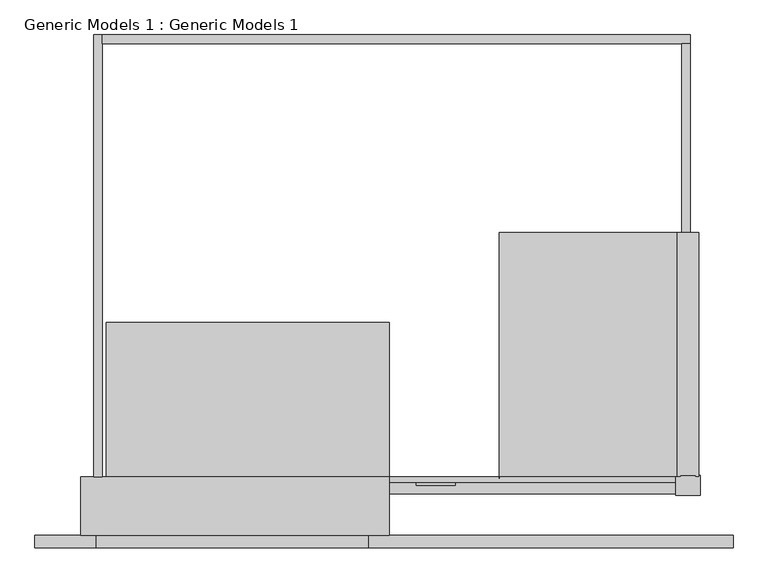
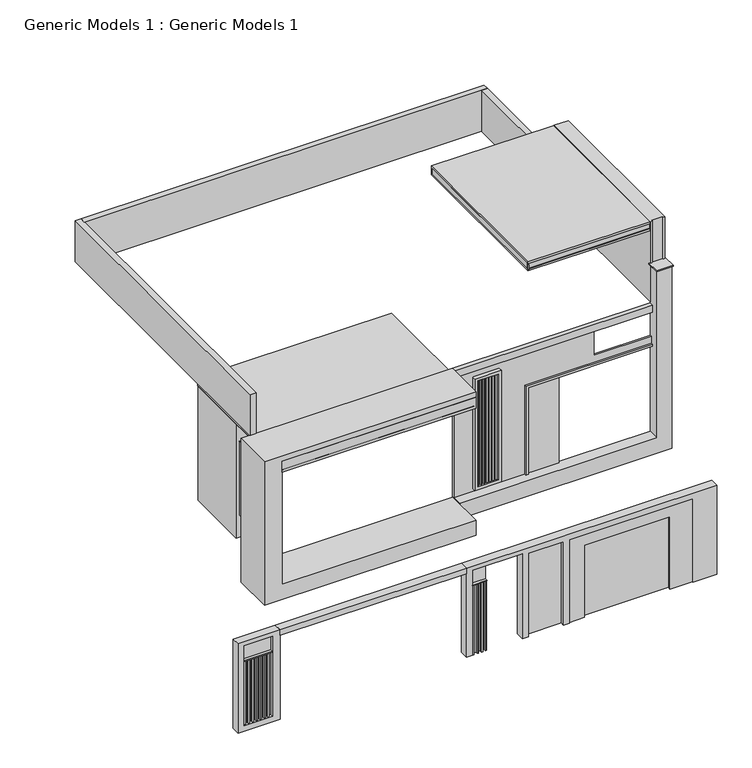
"""IFC4 building model written with IfcOpenShell, lengths in millimetres: proxy geometry, Generic Models 1 : Generic Models 1."""

from ifc_helpers import new_model, si_unit, frame, origin, place, context, project, spatial, polyline, outline, extrude, faceted_brep, source, transform, mapped, element, save


def generic_models_1_generic_models_1_ed2606db(model_context):
    return source(origin(), model_context, "Body", "SolidModel", [
        extrude(outline(polyline([(301.4620146, -6969.590216), (-1912.2392038, -6969.590216), (-1912.2392038, -6967.3081848), (301.4620146, -6967.3081848), (301.4620146, -6969.590216)])), frame((0.0, 0.0, -303.2125), z_axis=(0.0, 0.0, 1.0), x_axis=(1.0, 0.0, 0.0)), (0.0, 0.0, 1.0), 1981.2),
        extrude(outline(polyline([(-4450.5271999, -6992.7081848), (-4450.5271999, -7068.9081848), (-4829.3379854, -7068.9081848), (-4829.3379854, -6992.7081848), (-4450.5271999, -6992.7081848)])), frame((0.0, 0.0, 1601.8946299), z_axis=(0.0, 0.0, 1.0), x_axis=(1.0, 0.0, 0.0)), (0.0, 0.0, 1.0), 16.157027),
        extrude(outline(polyline([(-4784.1817029, -7018.3750374), (-4784.1817029, -7056.4750374), (-4815.9317029, -7056.4750374), (-4815.9317029, -7018.3750374), (-4784.1817029, -7018.3750374)])), frame((0.0, 0.0, -305.4945313), z_axis=(0.0, 0.0, 1.0), x_axis=(1.0, 0.0, 0.0)), (0.0, 0.0, 1.0), 1907.3891612),
        extrude(outline(polyline([(-4663.5317029, -7018.3750374), (-4663.5317029, -7056.4750374), (-4695.2817029, -7056.4750374), (-4695.2817029, -7018.3750374), (-4663.5317029, -7018.3750374)])), frame((0.0, 0.0, -305.4945313), z_axis=(0.0, 0.0, 1.0), x_axis=(1.0, 0.0, 0.0)), (0.0, 0.0, 1.0), 1907.3891612),
        extrude(outline(polyline([(-4555.5817029, -7018.3750374), (-4555.5817029, -7056.4750374), (-4587.3317029, -7056.4750374), (-4587.3317029, -7018.3750374), (-4555.5817029, -7018.3750374)])), frame((0.0, 0.0, -305.4945313), z_axis=(0.0, 0.0, 1.0), x_axis=(1.0, 0.0, 0.0)), (0.0, 0.0, 1.0), 1907.3891612),
        extrude(outline(polyline([(-4453.9817029, -7018.3750374), (-4453.9817029, -7056.4750374), (-4485.7317029, -7056.4750374), (-4485.7317029, -7018.3750374), (-4453.9817029, -7018.3750374)])), frame((0.0, 0.0, -305.4945313), z_axis=(0.0, 0.0, 1.0), x_axis=(1.0, 0.0, 0.0)), (0.0, 0.0, 1.0), 1907.3891612),
        extrude(outline(polyline([(-10010.9379854, -6992.7081848), (-10010.9379854, -7068.9081848), (-10747.5379854, -7068.9081848), (-10747.5379854, -6992.7081848), (-10010.9379854, -6992.7081848)])), frame((0.0, 0.0, 1597.653296), z_axis=(0.0, 0.0, 1.0), x_axis=(1.0, 0.0, 0.0)), (0.0, 0.0, 1.0), 20.398361),
        extrude(outline(polyline([(-10688.6480874, -7004.4126066), (-10688.6480874, -7048.8626066), (-10726.7480874, -7048.8626066), (-10726.7480874, -7004.4126066), (-10688.6480874, -7004.4126066)])), frame((0.0, 0.0, -152.4), z_axis=(0.0, 0.0, 1.0), x_axis=(1.0, 0.0, 0.0)), (0.0, 0.0, 1.0), 1750.053296),
        extrude(outline(polyline([(-10587.0480874, -7004.4126066), (-10587.0480874, -7048.8626066), (-10625.1480874, -7048.8626066), (-10625.1480874, -7004.4126066), (-10587.0480874, -7004.4126066)])), frame((0.0, 0.0, -152.4), z_axis=(0.0, 0.0, 1.0), x_axis=(1.0, 0.0, 0.0)), (0.0, 0.0, 1.0), 1750.053296),
        extrude(outline(polyline([(-10485.4480874, -7004.4126066), (-10485.4480874, -7048.8626066), (-10523.5480874, -7048.8626066), (-10523.5480874, -7004.4126066), (-10485.4480874, -7004.4126066)])), frame((0.0, 0.0, -152.4), z_axis=(0.0, 0.0, 1.0), x_axis=(1.0, 0.0, 0.0)), (0.0, 0.0, 1.0), 1750.053296),
        extrude(outline(polyline([(-10383.8480874, -7004.4126066), (-10383.8480874, -7048.8626066), (-10421.9480874, -7048.8626066), (-10421.9480874, -7004.4126066), (-10383.8480874, -7004.4126066)])), frame((0.0, 0.0, -152.4), z_axis=(0.0, 0.0, 1.0), x_axis=(1.0, 0.0, 0.0)), (0.0, 0.0, 1.0), 1750.053296),
        extrude(outline(polyline([(-10282.2480874, -7004.4126066), (-10282.2480874, -7048.8626066), (-10320.3480874, -7048.8626066), (-10320.3480874, -7004.4126066), (-10282.2480874, -7004.4126066)])), frame((0.0, 0.0, -152.4), z_axis=(0.0, 0.0, 1.0), x_axis=(1.0, 0.0, 0.0)), (0.0, 0.0, 1.0), 1750.053296),
        extrude(outline(polyline([(-10180.6480874, -7004.4126066), (-10180.6480874, -7048.8626066), (-10218.7480874, -7048.8626066), (-10218.7480874, -7004.4126066), (-10180.6480874, -7004.4126066)])), frame((0.0, 0.0, -152.4), z_axis=(0.0, 0.0, 1.0), x_axis=(1.0, 0.0, 0.0)), (0.0, 0.0, 1.0), 1750.053296),
        extrude(outline(polyline([(-10079.0480874, -7004.4126066), (-10079.0480874, -7048.8626066), (-10117.1480874, -7048.8626066), (-10117.1480874, -7004.4126066), (-10079.0480874, -7004.4126066)])), frame((0.0, 0.0, -152.4), z_axis=(0.0, 0.0, 1.0), x_axis=(1.0, 0.0, 0.0)), (0.0, 0.0, 1.0), 1750.053296),
        extrude(outline(polyline([(-4981.7379854, -6848.5250101), (-4981.7379854, -7068.9081848), (-9807.7379854, -7068.9081848), (-9807.7379854, -6848.5250101), (-4981.7379854, -6848.5250101)])), frame((0.0, 0.0, 1982.7875), z_axis=(0.0, 0.0, 1.0), x_axis=(1.0, 0.0, 0.0)), (0.0, 0.0, 1.0), 152.4),
        faceted_brep([(-10899.9379854, -6848.5250101, -303.2125), (-10899.9379854, -6848.5250101, 2135.1875), (-9807.7379854, -6848.5250101, 2135.1875), (-9807.7379854, -6848.5250101, -303.2125), (-10899.9379854, -7068.9081848, 2135.1875), (-10899.9379854, -7068.9081848, -303.2125), (-9807.7379854, -7068.9081848, -303.2125), (-9807.7379854, -7068.9081848, 2135.1875), (-10010.9379854, -7068.9081848, 2027.2375), (-10010.9379854, -7068.9081848, -152.4), (-10747.5379854, -7068.9081848, -152.4), (-10747.5379854, -7068.9081848, 2027.2375), (-10010.9379854, -6992.7081848, 2027.2375), (-10747.5379854, -6992.7081848, 2027.2375), (-10747.5379854, -6992.7081848, -152.4), (-10010.9379854, -6992.7081848, -152.4)], [[[0, 1, 2, 3]], [[4, 5, 6, 7], [8, 9, 10, 11]], [[5, 0, 3, 6]], [[1, 4, 7, 2]], [[1, 0, 5, 4]], [[12, 13, 14, 15]], [[12, 15, 9, 8]], [[15, 14, 10, 9]], [[14, 13, 11, 10]], [[13, 12, 8, 11]], [[3, 2, 7, 6]]]),
        faceted_brep([(1495.2620146, -6848.5250101, 2135.1875), (1495.2620146, -6848.5250101, -303.2125), (-3536.1271999, -6848.5250101, -303.2125), (-3536.1271999, -6848.5250101, 2027.2375), (-4450.5271999, -6848.5250101, 2027.2375), (-4450.5271999, -6848.5250101, -303.2125), (-4981.7379854, -6848.5250101, -303.2125), (-4981.7379854, -6848.5250101, 2135.1875), (1495.2620146, -7068.9081848, -303.2125), (1495.2620146, -7068.9081848, 2135.1875), (-4981.7379854, -7068.9081848, 2135.1875), (-4981.7379854, -7068.9081848, -303.2125), (-4829.3379854, -7068.9081848, -303.2125), (-4829.3379854, -7068.9081848, 2027.2375), (-3536.1271999, -7068.9081848, 2027.2375), (-3536.1271999, -7068.9081848, -303.2125), (-3385.4392038, -7068.9081848, -303.2125), (-3385.4392038, -7068.9081848, 1982.7875), (-2471.0392038, -7068.9081848, 1982.7875), (-2471.0392038, -7068.9081848, -303.2125), (-2318.6392038, -7068.9081848, -303.2125), (-2318.6392038, -7068.9081848, 1982.7875), (881.7607962, -7068.9081848, 1982.7875), (881.7607962, -7068.9081848, -303.2125), (881.7607962, -7043.5081848, -303.2125), (301.4620146, -7043.5081848, -303.2125), (301.4620146, -6967.3081848, -303.2125), (-1912.2392038, -6967.3081848, -303.2125), (-1912.2392038, -7043.5081848, -303.2125), (-2318.6392038, -7043.5081848, -303.2125), (-2471.0392038, -6967.3081848, -303.2125), (-3385.4392038, -6967.3081848, -303.2125), (-4450.5271999, -6992.7081848, -303.2125), (-4829.3379854, -6992.7081848, -303.2125), (-4450.5271999, -6992.7081848, 2027.2375), (-4829.3379854, -6992.7081848, 2027.2375), (-2471.0392038, -6967.3081848, 1982.7875), (-3385.4392038, -6967.3081848, 1982.7875), (881.7607962, -7043.5081848, 1982.7875), (-2318.6392038, -7043.5081848, 1982.7875), (-1912.2392038, -7043.5081848, 1677.9875), (301.4620146, -7043.5081848, 1677.9875), (301.4620146, -6967.3081848, 1677.9875), (-1912.2392038, -6967.3081848, 1677.9875)], [[[0, 1, 2, 3, 4, 5, 6, 7]], [[8, 9, 10, 11, 12, 13, 14, 15, 16, 17, 18, 19, 20, 21, 22, 23]], [[1, 8, 23, 24, 25, 26, 27, 28, 29, 20, 19, 30, 31, 16, 15, 2]], [[11, 6, 5, 32, 33, 12]], [[1, 0, 9, 8]], [[9, 0, 7, 10]], [[7, 6, 11, 10]], [[34, 35, 33, 32]], [[33, 35, 13, 12]], [[14, 3, 2, 15]], [[4, 34, 32, 5]], [[36, 37, 31, 30]], [[18, 36, 30, 19]], [[37, 17, 16, 31]], [[37, 36, 18, 17]], [[38, 39, 29, 28, 40, 41, 25, 24]], [[38, 24, 23, 22]], [[29, 39, 21, 20]], [[39, 38, 22, 21]], [[42, 43, 27, 26]], [[43, 40, 28, 27]], [[43, 42, 41, 40]], [[41, 42, 26, 25]], [[35, 34, 4, 3, 14, 13]]]),
        extrude(outline(polyline([(580.8620146, 1889.7493179), (733.2620146, 1889.7493179), (733.2620146, -1473.2538577), (580.8620146, -1473.2538577), (580.8620146, 1889.7493179)])), frame((0.0, 0.0, 6705.6), z_axis=(0.0, 0.0, 1.0), x_axis=(1.0, 0.0, 0.0)), (0.0, 0.0, 1.0), 1120.7052027),
        extrude(outline(polyline([(733.2620146, 2042.1493179), (733.2620146, 1889.7493179), (-9706.1379854, 1889.7493179), (-9706.1379854, 2042.1493179), (733.2620146, 2042.1493179)])), frame((0.0, 0.0, 6705.6), z_axis=(0.0, 0.0, 1.0), x_axis=(1.0, 0.0, 0.0)), (0.0, 0.0, 1.0), 1120.7052027),
        extrude(outline(polyline([(479.2620146, -6136.6506821), (479.2620146, -5781.0506821), (911.0620146, -5781.0506821), (911.0620146, -6136.6506821), (479.2620146, -6136.6506821)])), frame((0.0, 0.0, 7763.807089), z_axis=(0.0, 0.0, 1.0), x_axis=(1.0, 0.0, 0.0)), (0.0, 0.0, 1.0), 25.4),
        extrude(outline(polyline([(-9706.1379854, 2042.1493179), (-9706.1379854, -5806.4506821), (-9858.5379854, -5806.4506821), (-9858.5379854, 2042.1493179), (-9706.1379854, 2042.1493179)])), frame((0.0, 0.0, 6705.6), z_axis=(0.0, 0.0, 1.0), x_axis=(1.0, 0.0, 0.0)), (0.0, 0.0, 1.0), 1120.7052027),
        extrude(outline(polyline([(-2659.9200166, -5839.8554554), (-2659.9200166, -1524.0538577), (-2657.6379854, -1524.0538577), (-2657.6379854, -5839.8554554), (-2659.9200166, -5839.8554554)])), frame((0.0, 0.0, 8737.6), z_axis=(0.0, 0.0, 1.0), x_axis=(1.0, 0.0, 0.0)), (0.0, 0.0, 1.0), 144.3956442),
        extrude(outline(polyline([(-5806.4506821, 8932.7956442), (-1473.2538577, 8932.7956442), (-1473.2538577, 8686.8), (-5806.4506821, 8686.8), (-5806.4506821, 8737.6), (-5781.0506821, 8737.6), (-5781.0506821, 8881.9956442), (-5806.4506821, 8881.9956442), (-5806.4506821, 8932.7956442)])), frame((-2657.6379854, 0.0, 0.0), z_axis=(1.0, 0.0, 0.0), x_axis=(0.0, 1.0, 0.0)), (0.0, 0.0, 1.0), 3152.821357),
        faceted_brep([(885.6620146, -5806.4506821, 6735.2893122), (885.6620146, -1473.2538577, 6735.2893122), (885.6620146, -1473.2538577, 8932.7956442), (885.6620146, -5806.4506821, 8932.7956442), (504.6620146, -5806.4506821, 6735.2893122), (504.6620146, -5806.4506821, 8932.7956442), (504.6620146, -1473.2538577, 8932.7956442), (504.6620146, -1473.2538577, 6735.2893122), (555.4620146, -5806.4506821, 8932.7956442), (555.4620146, -5781.0506821, 8932.7956442), (834.8620146, -5781.0506821, 8932.7956442), (834.8620146, -5806.4506821, 8932.7956442), (834.8620146, -5806.4506821, 7723.2672819), (555.4620146, -5806.4506821, 7723.2672819), (555.4620146, -5781.0506821, 7723.2672819), (834.8620146, -5781.0506821, 7723.2672819)], [[[0, 1, 2, 3]], [[4, 5, 6, 7]], [[1, 0, 4, 7]], [[2, 1, 7, 6]], [[3, 2, 6, 5, 8, 9, 10, 11]], [[0, 3, 11, 12, 13, 8, 5, 4]], [[14, 15, 10, 9]], [[14, 9, 8, 13]], [[10, 15, 12, 11]], [[15, 14, 13, 12]]]),
        extrude(outline(polyline([(-9483.0640572, -4798.2905844), (-9483.0640572, -4817.3405844), (-9502.1140572, -4817.3405844), (-9502.1140572, -4798.2905844), (-9483.0640572, -4798.2905844)])), frame((0.0, 0.0, 3816.8368126), z_axis=(0.0, 0.0, 1.0), x_axis=(1.0, 0.0, 0.0)), (0.0, 0.0, 1.0), 1981.2),
        extrude(outline(polyline([(-9406.8640572, -4798.2905844), (-9406.8640572, -4817.3405844), (-9425.9140572, -4817.3405844), (-9425.9140572, -4798.2905844), (-9406.8640572, -4798.2905844)])), frame((0.0, 0.0, 3816.8368126), z_axis=(0.0, 0.0, 1.0), x_axis=(1.0, 0.0, 0.0)), (0.0, 0.0, 1.0), 1981.2),
        extrude(outline(polyline([(-9330.6640572, -4798.2905844), (-9330.6640572, -4817.3405844), (-9349.7140572, -4817.3405844), (-9349.7140572, -4798.2905844), (-9330.6640572, -4798.2905844)])), frame((0.0, 0.0, 3816.8368126), z_axis=(0.0, 0.0, 1.0), x_axis=(1.0, 0.0, 0.0)), (0.0, 0.0, 1.0), 1981.2),
        extrude(outline(polyline([(-9254.4640572, -4798.2905844), (-9254.4640572, -4817.3405844), (-9273.5140572, -4817.3405844), (-9273.5140572, -4798.2905844), (-9254.4640572, -4798.2905844)])), frame((0.0, 0.0, 3816.8368126), z_axis=(0.0, 0.0, 1.0), x_axis=(1.0, 0.0, 0.0)), (0.0, 0.0, 1.0), 1981.2),
        extrude(outline(polyline([(-9178.2640572, -4798.2905844), (-9178.2640572, -4817.3405844), (-9197.3140572, -4817.3405844), (-9197.3140572, -4798.2905844), (-9178.2640572, -4798.2905844)])), frame((0.0, 0.0, 3816.8368126), z_axis=(0.0, 0.0, 1.0), x_axis=(1.0, 0.0, 0.0)), (0.0, 0.0, 1.0), 1981.2),
        extrude(outline(polyline([(-9102.0640572, -4798.2905844), (-9102.0640572, -4817.3405844), (-9121.1140572, -4817.3405844), (-9121.1140572, -4798.2905844), (-9102.0640572, -4798.2905844)])), frame((0.0, 0.0, 3816.8368126), z_axis=(0.0, 0.0, 1.0), x_axis=(1.0, 0.0, 0.0)), (0.0, 0.0, 1.0), 1981.2),
        extrude(outline(polyline([(5823.4368126, -9039.0248121), (5823.4368126, -9547.0248121), (3791.4368126, -9547.0248121), (3791.4368126, -9039.0248121), (5823.4368126, -9039.0248121)]), holes=[polyline([(5798.0368126, -9064.4248121), (3816.8368126, -9064.4248121), (3816.8368126, -9521.6248121), (5798.0368126, -9521.6248121), (5798.0368126, -9064.4248121)])]), frame((0.0, -4832.6959633, 0.0), z_axis=(0.0, 1.0, 0.0), x_axis=(0.0, 0.0, 1.0)), (0.0, 0.0, 1.0), 50.8),
        extrude(outline(polyline([(-4664.2379854, -3063.2506821), (-4664.2379854, -6848.5250101), (-9629.9379854, -6848.5250101), (-9629.9379854, -3063.2506821), (-4664.2379854, -3063.2506821)])), frame((0.0, 0.0, 6322.3179687), z_axis=(0.0, 0.0, 1.0), x_axis=(1.0, 0.0, 0.0)), (0.0, 0.0, 1.0), 2.2820312),
        faceted_brep([(-4613.4379854, -3063.2506821, 6248.4), (-4613.4379854, -6848.5250101, 6248.4), (-9629.9379854, -6848.5250101, 6248.4), (-9629.9379854, -6797.7250101, 6248.4), (-4664.2379854, -6797.7250101, 6248.4), (-4664.2379854, -3063.2506821, 6248.4), (-9629.9379854, -6848.5250101, 6553.2), (-4613.4379854, -6848.5250101, 6553.2), (-4613.4379854, -3063.2506821, 6553.2), (-9629.9379854, -3063.2506821, 6553.2), (-9629.9379854, -3063.2506821, 6324.6), (-9629.9379854, -6797.7250101, 6324.6), (-4664.2379854, -3063.2506821, 6324.6), (-4664.2379854, -6797.7250101, 6324.6)], [[[0, 1, 2, 3, 4, 5]], [[6, 7, 8, 9]], [[6, 9, 10, 11, 3, 2]], [[9, 8, 0, 5, 12, 10]], [[1, 0, 8, 7]], [[2, 1, 7, 6]], [[12, 13, 11, 10]], [[11, 13, 4, 3]], [[13, 12, 5, 4]]]),
        faceted_brep([(-10089.7982204, -6848.5250101, 2776.4354451), (-4613.4379854, -6848.5250101, 2776.4354451), (-4613.4379854, -6848.5250101, 3182.8354451), (-9629.9379854, -6848.5250101, 3182.8354451), (-9629.9379854, -6848.5250101, 6299.2), (-4613.4379854, -6848.5250101, 6299.2), (-4613.4379854, -6848.5250101, 6705.6), (-10089.7982204, -6848.5250101, 6705.6), (-10089.7982204, -5806.4506821, 2776.4354451), (-10089.7982204, -5806.4506821, 6705.6), (-4613.4379854, -5806.4506821, 6705.6), (-4613.4379854, -5806.4506821, 6299.2), (-4664.2379854, -5806.4506821, 6299.2), (-4664.2379854, -5806.4506821, 6324.6), (-9629.9379854, -5806.4506821, 6324.6), (-9629.9379854, -5806.4506821, 3182.8354451), (-4613.4379854, -5806.4506821, 3182.8354451), (-4613.4379854, -5806.4506821, 2776.4354451), (-9629.9379854, -6797.7250101, 6324.6), (-9629.9379854, -6797.7250101, 6299.2), (-4664.2379854, -6797.7250101, 6299.2), (-4664.2379854, -6797.7250101, 6324.6)], [[[0, 1, 2, 3, 4, 5, 6, 7]], [[8, 9, 10, 11, 12, 13, 14, 15, 16, 17]], [[1, 0, 8, 17]], [[2, 1, 17, 16]], [[3, 2, 16, 15]], [[4, 3, 15, 14, 18, 19]], [[5, 4, 19, 20, 12, 11]], [[6, 5, 11, 10]], [[7, 6, 10, 9]], [[0, 7, 9, 8]], [[21, 18, 14, 13]], [[18, 21, 20, 19]], [[21, 13, 12, 20]]]),
        extrude(outline(polyline([(-8944.1379854, -3080.0959633), (-8944.1379854, -4781.8959633), (-9629.9379854, -4781.8959633), (-9629.9379854, -3080.0959633), (-8944.1379854, -3080.0959633)])), frame((0.0, 0.0, 3200.4), z_axis=(0.0, 0.0, 1.0), x_axis=(1.0, 0.0, 0.0)), (0.0, 0.0, 1.0), 3121.9179688),
        extrude(outline(polyline([(504.6620146, -5908.0506821), (-4613.4379854, -5908.0506821), (-4613.4379854, -5806.4506821), (504.6620146, -5806.4506821), (504.6620146, -5908.0506821)])), frame((0.0, 0.0, 6510.8201114), z_axis=(0.0, 0.0, 1.0), x_axis=(1.0, 0.0, 0.0)), (0.0, 0.0, 1.0), 194.7798886),
        extrude(outline(polyline([(7763.807089, 504.6620146), (3200.4, 504.6620146), (3200.4, -4600.7379854), (2776.4354451, -4600.7379854), (2776.4354451, 885.6620146), (7763.807089, 885.6620146), (7763.807089, 504.6620146)])), frame((0.0, -6111.2506821, 0.0), z_axis=(0.0, 1.0, 0.0), x_axis=(0.0, 0.0, 1.0)), (0.0, 0.0, 1.0), 304.8),
        extrude(outline(polyline([(3200.4, -2712.2511428), (5575.3, -2712.2511428), (5575.3, 504.6620146), (5638.8, 504.6620146), (5638.8, -2775.7511428), (3200.4, -2775.7511428), (3200.4, -2712.2511428)])), frame((0.0, -5908.0506821, 0.0), z_axis=(0.0, 1.0, 0.0), x_axis=(0.0, 0.0, 1.0)), (0.0, 0.0, 1.0), 50.8),
        extrude(outline(polyline([(-3995.9496056, -5890.0107026), (-3995.9496056, -5921.7607026), (-4027.6996056, -5921.7607026), (-4027.6996056, -5890.0107026), (-3995.9496056, -5890.0107026)])), frame((0.0, 0.0, 3362.1943504), z_axis=(0.0, 0.0, 1.0), x_axis=(1.0, 0.0, 0.0)), (0.0, 0.0, 1.0), 2895.6),
        extrude(outline(polyline([(-3919.7496056, -5890.0107026), (-3919.7496056, -5921.7607026), (-3951.4996056, -5921.7607026), (-3951.4996056, -5890.0107026), (-3919.7496056, -5890.0107026)])), frame((0.0, 0.0, 3362.1943504), z_axis=(0.0, 0.0, 1.0), x_axis=(1.0, 0.0, 0.0)), (0.0, 0.0, 1.0), 2895.6),
        extrude(outline(polyline([(-3843.5496056, -5890.0107026), (-3843.5496056, -5921.7607026), (-3875.2996056, -5921.7607026), (-3875.2996056, -5890.0107026), (-3843.5496056, -5890.0107026)])), frame((0.0, 0.0, 3362.1943504), z_axis=(0.0, 0.0, 1.0), x_axis=(1.0, 0.0, 0.0)), (0.0, 0.0, 1.0), 2895.6),
        extrude(outline(polyline([(-3767.3496056, -5890.0107026), (-3767.3496056, -5921.7607026), (-3799.0996056, -5921.7607026), (-3799.0996056, -5890.0107026), (-3767.3496056, -5890.0107026)])), frame((0.0, 0.0, 3362.1943504), z_axis=(0.0, 0.0, 1.0), x_axis=(1.0, 0.0, 0.0)), (0.0, 0.0, 1.0), 2895.6),
        extrude(outline(polyline([(-3691.1496056, -5890.0107026), (-3691.1496056, -5921.7607026), (-3722.8996056, -5921.7607026), (-3722.8996056, -5890.0107026), (-3691.1496056, -5890.0107026)])), frame((0.0, 0.0, 3362.1943504), z_axis=(0.0, 0.0, 1.0), x_axis=(1.0, 0.0, 0.0)), (0.0, 0.0, 1.0), 2895.6),
        extrude(outline(polyline([(-3614.9496056, -5890.0107026), (-3614.9496056, -5921.7607026), (-3646.6996056, -5921.7607026), (-3646.6996056, -5890.0107026), (-3614.9496056, -5890.0107026)])), frame((0.0, 0.0, 3362.1943504), z_axis=(0.0, 0.0, 1.0), x_axis=(1.0, 0.0, 0.0)), (0.0, 0.0, 1.0), 2895.6),
        extrude(outline(polyline([(-3538.7496056, -5890.0107026), (-3538.7496056, -5921.7607026), (-3570.4996056, -5921.7607026), (-3570.4996056, -5890.0107026), (-3538.7496056, -5890.0107026)])), frame((0.0, 0.0, 3362.1943504), z_axis=(0.0, 0.0, 1.0), x_axis=(1.0, 0.0, 0.0)), (0.0, 0.0, 1.0), 2895.6),
        extrude(outline(polyline([(6333.9943504, -3440.0190446), (6333.9943504, -4125.8190446), (3285.9943504, -4125.8190446), (3285.9943504, -3440.0190446), (6333.9943504, -3440.0190446)]), holes=[polyline([(6257.7943504, -3516.2190446), (3362.1943504, -3516.2190446), (3362.1943504, -4049.6190446), (6257.7943504, -4049.6190446), (6257.7943504, -3516.2190446)])]), frame((0.0, -5958.8506821, 0.0), z_axis=(0.0, 1.0, 0.0), x_axis=(0.0, 0.0, 1.0)), (0.0, 0.0, 1.0), 101.6),
        extrude(outline(polyline([(6510.8201114, -979.002741), (6510.8201114, -4613.4379854), (3200.4, -4613.4379854), (3200.4, -1893.402741), (5571.9943504, -1893.402741), (5571.9943504, 504.6620146), (5825.9943504, 504.6620146), (5825.9943504, -979.002741), (6510.8201114, -979.002741)])), frame((0.0, -5857.2506821, 0.0), z_axis=(0.0, 1.0, 0.0), x_axis=(0.0, 0.0, 1.0)), (0.0, 0.0, 1.0), 50.8),
    ])


if __name__ == "__main__":
    model = new_model("IFC4")
    model_context = context("Model", 3, world=origin())
    ifc_project = project(units=[si_unit("LENGTHUNIT", "METRE", prefix="MILLI")], contexts=[model_context])
    site = spatial("IfcSite", under=ifc_project)
    building = spatial("IfcBuilding", under=site)
    placement = place(None, origin())
    generic_models_1_generic_models_1_shape = generic_models_1_generic_models_1_ed2606db(model_context)
    element("IfcBuildingElementProxy", 1, Name="Generic Models 1 : Generic Models 1", ObjectType="Generic Models 1 : Generic Models 1", at=placement, inside=building, context=model_context, shape_type="MappedRepresentation", body=[
        mapped(generic_models_1_generic_models_1_shape, transform((0.0, 0.0, 0.0), x_axis=(1.0, 0.0, 0.0), y_axis=(0.0, 1.0, 0.0), z_axis=(0.0, 0.0, 1.0))),
    ])
    save(model, "model.ifc")

# Revit data of these elements
# Element 1 (IfcBuildingElementProxy, "Generic Models 1 : Generic Models 1")
#   Materials on its faces: "door", "Wood - Stained", "balcony wall", "mullions", "black"
# Materials
#   "door": class "Generic", colour RGB 120 120 120, transparency 0, Cost = 0
#   "Wood - Stained": class "Wood", colour RGB 224 178 126, transparency 0, Cost = 0
#   "balcony wall": class "Generic", colour RGB 120 120 120, transparency 0, Cost = 0
#   "mullions": class "Generic", colour RGB 120 120 120, transparency 0, Cost = 0
#   "black": class "Generic", colour RGB 120 120 120, transparency 0, Cost = 0
